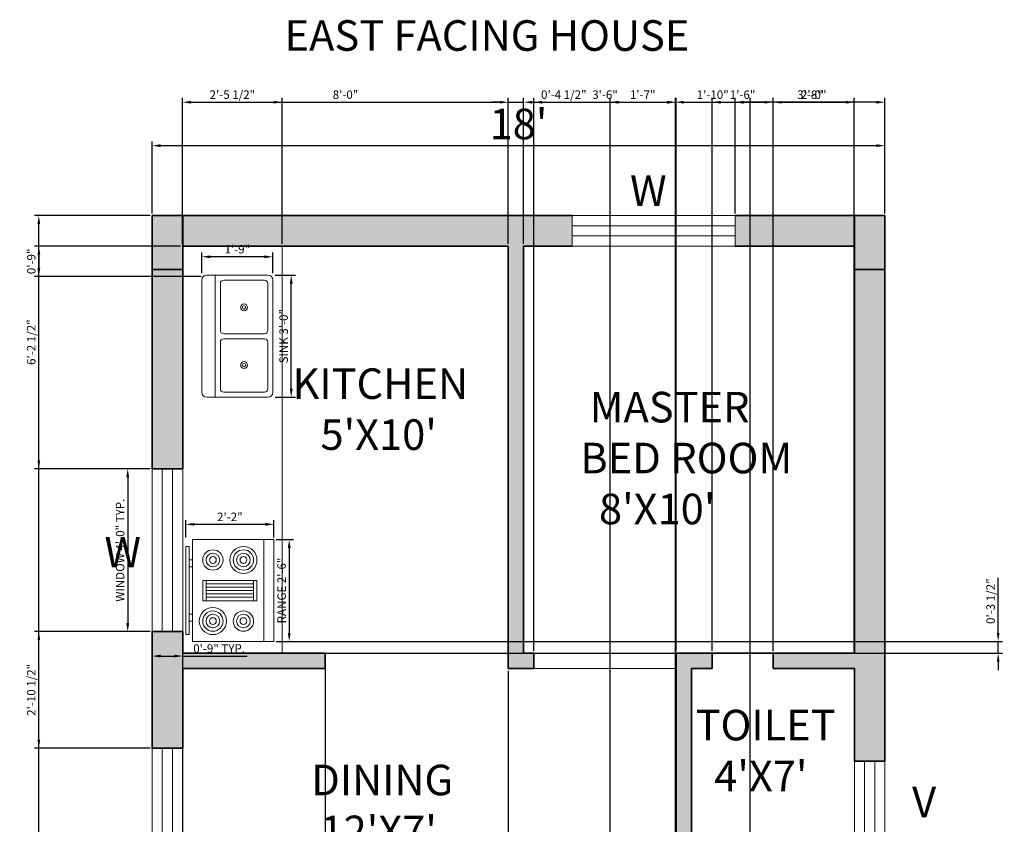
# Model space of a CAD drawing. Units: inches. Extents: x 4888 to 5178, y 5041 to 5743.
# Tile 3 of 3: x 4888 to 5178, y 5506 to 5743. Entities that reach past the tile are written whole.
import ezdxf

# ---------------------------------------------------------------- set-up
doc = ezdxf.new("R2010")
doc.units = ezdxf.units.IN
for name, color, linetype, lineweight in [('A-ANNO-DIMS', 2, 'Continuous', 18), ('A-ANNO-TEXT', 7, 'Continuous', 18), ('A-AREA-IDEN', 7, 'Continuous', 18), ('A-COLS', 7, 'Continuous', 35), ('A-DOOR', 4, 'Continuous', 18), ('A-EQPM', 9, 'Continuous', 18), ('A-FLOR-CASE', 9, 'Continuous', 18), ('A-FLOR-FIXT', 9, 'Continuous', 18), ('A-WALL', 7, 'Continuous', 35), ('A-WALL-PATT', 8, 'Continuous', 13)]:
    doc.layers.add(name, color=color, linetype=linetype, lineweight=lineweight)
doc.layers.add('A-COLS-PATT', color=18, linetype='Continuous', lineweight=13, true_color=0x000000)
doc.layers.add('A-GLAZ', color=31, linetype='Continuous', lineweight=18, true_color=0xfecc66)
doc.styles.get("Standard").update_dxf_attribs({"font": 'arial.ttf'})
doc.dimstyles.new('ISO-25', dxfattribs={"dimtxt": 2.5, "dimasz": 2.5, "dimexe": 1.25, "dimexo": 0.625, "dimtad": 1, "dimlunit": 3, "dimtxsty": 'Standard', "dimcen": 2.5, "dimadec": 0, "dimazin": 0, "dimtfac": 1, "dimtmove": 0, "dimatfit": 3, "dimfxl": 1, "dimarcsym": 0})

# ---------------------------------------------------------------- blocks, each defined once
blk = doc.blocks.new('*D1')
at = {"layer": 'A-ANNO-DIMS', "color": 0, "lineweight": -2, "transparency": 16777216}
for p, q in [((4926.84, 5685.63), (4926.84, 5706.86)), ((5142.84, 5685.63), (5142.84, 5706.86)), ((4929.34, 5705.61), (5140.34, 5705.61))]:
    blk.add_line(p, q, dxfattribs=at)
at = {"layer": 'A-ANNO-DIMS', "color": 0, "transparency": 16777216}
for points in [[(4929.34, 5706.02), (4929.34, 5705.19), (4926.84, 5705.61)], [(5140.34, 5706.02), (5140.34, 5705.19), (5142.84, 5705.61)]]:
    blk.add_solid(points, dxfattribs=at)
at = {"layer": 'Defpoints', "color": 0, "transparency": 16777216}
for p in [(5142.84, 5705.61), (4926.84, 5685.01), (5142.84, 5685.01)]:
    blk.add_point(p, dxfattribs=at)
at = {"layer": 'A-ANNO-DIMS', "color": 0, "transparency": 16777216, "insert": (5034.84, 5710.83), "char_height": 9, "attachment_point": 5}
blk.add_mtext("18'", dxfattribs=at)
blk = doc.blocks.new('Range-Oven - 30 in top')
for p, q in [((0, -3), (30, -3)), ((12, -6), (18, -6)), ((13, -20), (13, -6)), ((14, -6), (14, -20)), ((15, -20), (15, -6)), ((16, -6), (16, -20)), ((17, -20), (17, -6)), ((18, -20), (12, -20)), ((6, -24), (6, -25)), ((8, -25), (8, -24)), ((22, -25), (22, -24)), ((24, -24), (24, -25))]:
    blk.add_line(p, q)
for points in [[(0, -24), (0, 0), (30, 0), (30, -24)], [(12, -21), (12, -5), (18, -5), (18, -21)], [(2, -26), (2, -25), (28, -25), (28, -26)]]:
    blk.add_lwpolyline(points, close=True)
for centre, radius in [((6, -9), 4), ((6, -9), 3), ((6, -9), 2), ((6, -9), 1), ((24, -9), 3), ((24, -9), 2), ((24, -9), 1), ((24, -18), 4), ((6, -18), 3), ((6, -18), 2), ((6, -18), 1), ((24, -18), 3), ((24, -18), 2), ((24, -18), 1)]:
    blk.add_circle(centre, radius)
blk = doc.blocks.new('Sink-double - 36 in top')
for p, q in [((-18, -4), (18, -4)), ((-0.75, -18.5), (-0.75, -6.5)), ((0.75, -6.5), (0.75, -18.5))]:
    blk.add_line(p, q)
for points in [[(-16.5, 0), (16.5, 0)], [(-18, -19.5), (-18, -1.5)], [(18, -1.5), (18, -19.5)], [(-15.5, -5.5), (-1.75, -5.5)], [(1.75, -5.5), (15.5, -5.5)], [(-16.5, -18.5), (-16.5, -6.5)], [(16.5, -6.5), (16.5, -18.5)], [(-1.75, -19.5), (-15.5, -19.5)], [(15.5, -19.5), (1.75, -19.5)], [(16.5, -21), (-16.5, -21)]]:
    blk.add_lwpolyline(points)
for centre, radius in [((-8.5, -12.5), 1), ((8.5, -12.5), 1), ((-8.5, -12.5), 0.5), ((8.5, -12.5), 0.5)]:
    blk.add_circle(centre, radius)
for centre, radius, start, end in [((-16.5, -1.5), 1.5, 90, 180), ((16.5, -1.5), 1.5, 0, 90), ((-15.5, -6.5), 1, 90, 180), ((-1.75, -6.5), 1, 0, 90), ((1.75, -6.5), 1, 90, 180), ((15.5, -6.5), 1, 0, 90), ((-16.5, -19.5), 1.5, 180, 270), ((-15.5, -18.5), 1, 180, 270), ((-1.75, -18.5), 1, 270, 0), ((1.75, -18.5), 1, 180, 270), ((15.5, -18.5), 1, 270, 0), ((16.5, -19.5), 1.5, 270, 0)]:
    blk.add_arc(centre, radius, start, end)
blk = doc.blocks.new('WIN-48IN')
for p, q in [((0, 9), (0, 0)), ((48, 9), (0, 9)), ((48, 0), (48, 9)), ((48, 6), (0, 6)), ((48, 3), (0, 3)), ((0, 0), (48, 0))]:
    blk.add_line(p, q)
blk = doc.blocks.new('VENT-24IN')
for p, q in [((0, 24), (0, 0)), ((9, 24), (0, 24)), ((3, 0), (3, 24)), ((6, 0), (6, 24)), ((9, 0), (9, 24)), ((0, 0), (9, 0))]:
    blk.add_line(p, q)
blk = doc.blocks.new('*D7')
at = {"layer": 'A-ANNO-DIMS', "color": 0, "lineweight": -2, "transparency": 16777216}
for p, q in [((4926.22, 5610.4), (4918.39, 5610.4)), ((4919.64, 5607.9), (4919.64, 5564.9)), ((4926.22, 5562.4), (4918.39, 5562.4))]:
    blk.add_line(p, q, dxfattribs=at)
at = {"layer": 'A-ANNO-DIMS', "color": 0, "transparency": 16777216}
for points in [[(4919.23, 5607.9), (4920.06, 5607.9), (4919.64, 5610.4)], [(4919.23, 5564.9), (4920.06, 5564.9), (4919.64, 5562.4)]]:
    blk.add_solid(points, dxfattribs=at)
at = {"layer": 'Defpoints', "color": 0, "transparency": 16777216}
for p in [(4926.84, 5610.4), (4919.64, 5562.4), (4926.84, 5562.4)]:
    blk.add_point(p, dxfattribs=at)
at = {"layer": 'A-ANNO-DIMS', "color": 0, "transparency": 16777216, "insert": (4917.73, 5586.4), "char_height": 2.5, "attachment_point": 5, "rotation": 90}
blk.add_mtext('WINDOW 4\'-0" TYP.', dxfattribs=at)
blk = doc.blocks.new('*D8')
at = {"layer": 'A-ANNO-DIMS', "color": 0, "lineweight": -2, "transparency": 16777216}
for p, q in [((4926.84, 5561.78), (4926.84, 5553.95)), ((4935.84, 5561.78), (4935.84, 5553.95)), ((4929.34, 5555.2), (4933.34, 5555.2)), ((4935.84, 5555.2), (4954.83, 5555.2))]:
    blk.add_line(p, q, dxfattribs=at)
at = {"layer": 'A-ANNO-DIMS', "color": 0, "transparency": 16777216}
for points in [[(4929.34, 5555.62), (4929.34, 5554.78), (4926.84, 5555.2)], [(4933.34, 5555.62), (4933.34, 5554.78), (4935.84, 5555.2)]]:
    blk.add_solid(points, dxfattribs=at)
at = {"layer": 'Defpoints', "color": 0, "transparency": 16777216}
for p in [(4926.84, 5562.4), (4935.84, 5562.4), (4935.84, 5555.2)]:
    blk.add_point(p, dxfattribs=at)
at = {"layer": 'A-ANNO-DIMS', "color": 0, "transparency": 16777216, "insert": (4946.59, 5557.1), "char_height": 2.5, "attachment_point": 5}
blk.add_mtext('0\'-9" TYP.', dxfattribs=at)
blk = doc.blocks.new('*D13')
at = {"layer": 'A-ANNO-DIMS', "color": 0, "lineweight": -2, "transparency": 16777216}
for p, q in [((4963.38, 5589.52), (4968.5, 5589.52)), ((4967.25, 5587.02), (4967.25, 5562.02)), ((4963.38, 5559.52), (4968.5, 5559.52))]:
    blk.add_line(p, q, dxfattribs=at)
at = {"layer": 'A-ANNO-DIMS', "color": 0, "transparency": 16777216}
for points in [[(4966.83, 5587.02), (4967.67, 5587.02), (4967.25, 5589.52)], [(4966.83, 5562.02), (4967.67, 5562.02), (4967.25, 5559.52)]]:
    blk.add_solid(points, dxfattribs=at)
at = {"layer": 'Defpoints', "color": 0, "transparency": 16777216}
for p in [(4962.75, 5589.52), (4962.75, 5559.52), (4967.25, 5559.52)]:
    blk.add_point(p, dxfattribs=at)
at = {"layer": 'A-ANNO-DIMS', "color": 0, "transparency": 16777216, "insert": (4965.33, 5574.52), "char_height": 2.5, "attachment_point": 5, "rotation": 90}
blk.add_mtext('RANGE 2\'-6"', dxfattribs=at)
blk = doc.blocks.new('*D14')
at = {"layer": 'A-ANNO-DIMS', "color": 0, "lineweight": -2, "transparency": 16777216}
for p, q in [((4936.75, 5590.14), (4936.75, 5595.27)), ((4939.25, 5594.02), (4960.25, 5594.02)), ((4962.75, 5590.14), (4962.75, 5595.27))]:
    blk.add_line(p, q, dxfattribs=at)
at = {"layer": 'A-ANNO-DIMS', "color": 0, "transparency": 16777216}
for points in [[(4939.25, 5594.43), (4939.25, 5593.6), (4936.75, 5594.02)], [(4960.25, 5594.43), (4960.25, 5593.6), (4962.75, 5594.02)]]:
    blk.add_solid(points, dxfattribs=at)
at = {"layer": 'Defpoints', "color": 0, "transparency": 16777216}
for p in [(4962.75, 5594.02), (4936.75, 5589.52), (4962.75, 5589.52)]:
    blk.add_point(p, dxfattribs=at)
at = {"layer": 'A-ANNO-DIMS', "color": 0, "transparency": 16777216, "insert": (4949.75, 5595.9), "char_height": 2.5, "attachment_point": 5}
blk.add_mtext('2\'-2"', dxfattribs=at)
blk = doc.blocks.new('*D15')
at = {"layer": 'A-ANNO-DIMS', "color": 0, "lineweight": -2, "transparency": 16777216}
for p, q in [((4963.07, 5667.46), (4969.1, 5667.46)), ((4967.85, 5633.96), (4967.85, 5664.96)), ((4963.07, 5631.46), (4969.1, 5631.46))]:
    blk.add_line(p, q, dxfattribs=at)
at = {"layer": 'A-ANNO-DIMS', "color": 0, "transparency": 16777216}
for points in [[(4967.43, 5664.96), (4968.26, 5664.96), (4967.85, 5667.46)], [(4967.43, 5633.96), (4968.26, 5633.96), (4967.85, 5631.46)]]:
    blk.add_solid(points, dxfattribs=at)
at = {"layer": 'Defpoints', "color": 0, "transparency": 16777216}
for p in [(4962.45, 5667.46), (4967.85, 5667.46), (4962.45, 5631.46)]:
    blk.add_point(p, dxfattribs=at)
at = {"layer": 'A-ANNO-DIMS', "color": 0, "transparency": 16777216, "insert": (4965.93, 5649.46), "char_height": 2.5, "attachment_point": 5, "rotation": 90}
blk.add_mtext('SINK 3\'-0"', dxfattribs=at)
blk = doc.blocks.new('*D16')
at = {"layer": 'A-ANNO-DIMS', "color": 0, "lineweight": -2, "transparency": 16777216}
for p, q in [((4941.45, 5668.08), (4941.45, 5674.11)), ((4959.95, 5672.86), (4943.95, 5672.86)), ((4962.45, 5668.08), (4962.45, 5674.11))]:
    blk.add_line(p, q, dxfattribs=at)
at = {"layer": 'A-ANNO-DIMS', "color": 0, "transparency": 16777216}
for points in [[(4943.95, 5673.27), (4943.95, 5672.44), (4941.45, 5672.86)], [(4959.95, 5673.27), (4959.95, 5672.44), (4962.45, 5672.86)]]:
    blk.add_solid(points, dxfattribs=at)
at = {"layer": 'Defpoints', "color": 0, "transparency": 16777216}
for p in [(4941.45, 5672.86), (4941.45, 5667.46), (4962.45, 5667.46)]:
    blk.add_point(p, dxfattribs=at)
at = {"layer": 'A-ANNO-DIMS', "color": 0, "transparency": 16777216, "insert": (4951.95, 5674.76), "char_height": 2.5, "attachment_point": 5}
blk.add_mtext('1\'-9"', dxfattribs=at)
blk = doc.blocks.new('*D17')
at = {"layer": 'A-ANNO-DIMS', "color": 0, "lineweight": -2, "transparency": 16777216}
for p, q in [((4926.22, 5685.01), (4892.19, 5685.01)), ((4893.44, 5078.51), (4893.44, 5682.51)), ((4926.22, 5076.01), (4892.19, 5076.01))]:
    blk.add_line(p, q, dxfattribs=at)
at = {"layer": 'A-ANNO-DIMS', "color": 0, "transparency": 16777216}
for points in [[(4893.03, 5682.51), (4893.86, 5682.51), (4893.44, 5685.01)], [(4893.03, 5078.51), (4893.86, 5078.51), (4893.44, 5076.01)]]:
    blk.add_solid(points, dxfattribs=at)
at = {"layer": 'Defpoints', "color": 0, "transparency": 16777216}
for p in [(4893.44, 5685.01), (4926.84, 5685.01), (4926.84, 5076.01)]:
    blk.add_point(p, dxfattribs=at)
at = {"layer": 'A-ANNO-DIMS', "color": 0, "transparency": 16777216, "insert": (4891.54, 5380.51), "char_height": 2.5, "attachment_point": 5, "rotation": 90}
blk.add_mtext('50\'-9"', dxfattribs=at)
blk = doc.blocks.new('*D18')
at = {"layer": 'A-ANNO-DIMS', "color": 0, "lineweight": -2, "transparency": 16777216}
for p, q in [((5098.68, 5685.63), (5098.68, 5719.66)), ((5140.34, 5718.41), (5101.18, 5718.41)), ((5142.84, 5685.63), (5142.84, 5719.66))]:
    blk.add_line(p, q, dxfattribs=at)
at = {"layer": 'A-ANNO-DIMS', "color": 0, "transparency": 16777216}
for points in [[(5101.18, 5718.82), (5101.18, 5717.99), (5098.68, 5718.41)], [(5140.34, 5718.82), (5140.34, 5717.99), (5142.84, 5718.41)]]:
    blk.add_solid(points, dxfattribs=at)
at = {"layer": 'Defpoints', "color": 0, "transparency": 16777216}
for p in [(5098.68, 5718.41), (5098.68, 5685.01), (5142.84, 5685.01)]:
    blk.add_point(p, dxfattribs=at)
at = {"layer": 'A-ANNO-DIMS', "color": 0, "transparency": 16777216, "insert": (5120.76, 5720.31), "char_height": 2.5, "attachment_point": 5}
blk.add_mtext('3\'-8"', dxfattribs=at)
blk = doc.blocks.new('*D19')
at = {"layer": 'A-ANNO-DIMS', "color": 0, "lineweight": -2, "transparency": 16777216}
for p, q in [((4926.22, 5685.01), (4892.19, 5685.01)), ((4893.44, 5612.9), (4893.44, 5682.51)), ((4926.22, 5610.4), (4892.19, 5610.4))]:
    blk.add_line(p, q, dxfattribs=at)
at = {"layer": 'A-ANNO-DIMS', "color": 0, "transparency": 16777216}
for points in [[(4893.03, 5682.51), (4893.86, 5682.51), (4893.44, 5685.01)], [(4893.03, 5612.9), (4893.86, 5612.9), (4893.44, 5610.4)]]:
    blk.add_solid(points, dxfattribs=at)
at = {"layer": 'Defpoints', "color": 0, "transparency": 16777216}
for p in [(4893.44, 5685.01), (4926.84, 5685.01), (4926.84, 5610.4)]:
    blk.add_point(p, dxfattribs=at)
at = {"layer": 'A-ANNO-DIMS', "color": 0, "transparency": 16777216, "insert": (4891.53, 5647.7), "char_height": 2.5, "attachment_point": 5, "rotation": 90}
blk.add_mtext('6\'-2 1/2"', dxfattribs=at)
blk = doc.blocks.new('*D20')
at = {"layer": 'A-ANNO-DIMS', "color": 0, "lineweight": -2, "transparency": 16777216}
for p, q in [((4926.22, 5562.4), (4892.19, 5562.4)), ((4893.44, 5530.6), (4893.44, 5559.9)), ((4926.22, 5528.1), (4892.19, 5528.1))]:
    blk.add_line(p, q, dxfattribs=at)
at = {"layer": 'A-ANNO-DIMS', "color": 0, "transparency": 16777216}
for points in [[(4893.03, 5559.9), (4893.86, 5559.9), (4893.44, 5562.4)], [(4893.03, 5530.6), (4893.86, 5530.6), (4893.44, 5528.1)]]:
    blk.add_solid(points, dxfattribs=at)
at = {"layer": 'Defpoints', "color": 0, "transparency": 16777216}
for p in [(4893.44, 5562.4), (4926.84, 5562.4), (4926.84, 5528.1)]:
    blk.add_point(p, dxfattribs=at)
at = {"layer": 'A-ANNO-DIMS', "color": 0, "transparency": 16777216, "insert": (4891.53, 5545.25), "char_height": 2.5, "attachment_point": 5, "rotation": 90}
blk.add_mtext('2\'-10 1/2"', dxfattribs=at)
blk = doc.blocks.new('*D32')
at = {"layer": 'A-ANNO-DIMS', "color": 0, "lineweight": -2, "transparency": 16777216}
for p, q in [((4977.89, 5550.88), (4977.89, 5041.36)), ((5031.84, 5550.88), (5031.84, 5041.36)), ((4980.39, 5042.61), (5029.34, 5042.61))]:
    blk.add_line(p, q, dxfattribs=at)
at = {"layer": 'A-ANNO-DIMS', "color": 0, "transparency": 16777216}
for points in [[(4980.39, 5043.02), (4980.39, 5042.19), (4977.89, 5042.61)], [(5029.34, 5043.02), (5029.34, 5042.19), (5031.84, 5042.61)]]:
    blk.add_solid(points, dxfattribs=at)
at = {"layer": 'Defpoints', "color": 0, "transparency": 16777216}
for p in [(4977.89, 5551.51), (5031.84, 5551.51), (5031.84, 5042.61)]:
    blk.add_point(p, dxfattribs=at)
at = {"layer": 'A-ANNO-DIMS', "color": 0, "transparency": 16777216, "insert": (5004.87, 5044.51), "char_height": 2.5, "attachment_point": 5}
blk.add_mtext('4\'-6"', dxfattribs=at)
blk = doc.blocks.new('*D33')
at = {"layer": 'A-ANNO-DIMS', "color": 0, "lineweight": -2, "transparency": 16777216}
for p, q in [((5039.34, 5556.63), (5039.34, 5719.66)), ((5041.84, 5718.41), (5078.84, 5718.41)), ((5081.34, 5556.63), (5081.34, 5719.66))]:
    blk.add_line(p, q, dxfattribs=at)
at = {"layer": 'A-ANNO-DIMS', "color": 0, "transparency": 16777216}
for points in [[(5041.84, 5718.82), (5041.84, 5717.99), (5039.34, 5718.41)], [(5078.84, 5718.82), (5078.84, 5717.99), (5081.34, 5718.41)]]:
    blk.add_solid(points, dxfattribs=at)
at = {"layer": 'Defpoints', "color": 0, "transparency": 16777216}
for p in [(5081.34, 5718.41), (5039.34, 5556.01), (5081.34, 5556.01)]:
    blk.add_point(p, dxfattribs=at)
at = {"layer": 'A-ANNO-DIMS', "color": 0, "transparency": 16777216, "insert": (5060.34, 5720.31), "char_height": 2.5, "attachment_point": 5}
blk.add_mtext('3\'-6"', dxfattribs=at)
blk = doc.blocks.new('*D34')
at = {"layer": 'A-ANNO-DIMS', "color": 0, "lineweight": -2, "transparency": 16777216}
for p, q in [((5091.9, 5556.63), (5091.9, 5719.66)), ((5094.4, 5718.41), (5107.4, 5718.41)), ((5109.9, 5556.63), (5109.9, 5719.66))]:
    blk.add_line(p, q, dxfattribs=at)
at = {"layer": 'A-ANNO-DIMS', "color": 0, "transparency": 16777216}
for points in [[(5094.4, 5718.82), (5094.4, 5717.99), (5091.9, 5718.41)], [(5107.4, 5718.82), (5107.4, 5717.99), (5109.9, 5718.41)]]:
    blk.add_solid(points, dxfattribs=at)
at = {"layer": 'Defpoints', "color": 0, "transparency": 16777216}
for p in [(5109.9, 5718.41), (5091.9, 5556.01), (5109.9, 5556.01)]:
    blk.add_point(p, dxfattribs=at)
at = {"layer": 'A-ANNO-DIMS', "color": 0, "transparency": 16777216, "insert": (5100.9, 5720.31), "char_height": 2.5, "attachment_point": 5}
blk.add_mtext('1\'-6"', dxfattribs=at)
blk = doc.blocks.new('*D35')
at = {"layer": 'A-ANNO-DIMS', "color": 0, "lineweight": -2, "transparency": 16777216}
for p, q in [((5109.9, 5556.63), (5109.9, 5719.66)), ((5112.4, 5718.41), (5131.34, 5718.41)), ((5133.84, 5556.63), (5133.84, 5719.66))]:
    blk.add_line(p, q, dxfattribs=at)
at = {"layer": 'A-ANNO-DIMS', "color": 0, "transparency": 16777216}
for points in [[(5112.4, 5718.82), (5112.4, 5717.99), (5109.9, 5718.41)], [(5131.34, 5718.82), (5131.34, 5717.99), (5133.84, 5718.41)]]:
    blk.add_solid(points, dxfattribs=at)
at = {"layer": 'Defpoints', "color": 0, "transparency": 16777216}
for p in [(5133.84, 5718.41), (5109.9, 5556.01), (5133.84, 5556.01)]:
    blk.add_point(p, dxfattribs=at)
at = {"layer": 'A-ANNO-DIMS', "color": 0, "transparency": 16777216, "insert": (5121.87, 5720.31), "char_height": 2.5, "attachment_point": 5}
blk.add_mtext('2\'-0"', dxfattribs=at)
blk = doc.blocks.new('*D36')
at = {"layer": 'A-ANNO-DIMS', "color": 0, "lineweight": -2, "transparency": 16777216}
for p, q in [((5081.08, 5204.13), (5081.08, 5719.66)), ((5083.58, 5718.41), (5100.61, 5718.41)), ((5103.11, 5204.13), (5103.11, 5719.66))]:
    blk.add_line(p, q, dxfattribs=at)
at = {"layer": 'A-ANNO-DIMS', "color": 0, "transparency": 16777216}
for points in [[(5083.58, 5718.82), (5083.58, 5717.99), (5081.08, 5718.41)], [(5100.61, 5718.82), (5100.61, 5717.99), (5103.11, 5718.41)]]:
    blk.add_solid(points, dxfattribs=at)
at = {"layer": 'Defpoints', "color": 0, "transparency": 16777216}
for p in [(5103.11, 5718.41), (5081.08, 5203.51), (5103.11, 5203.51)]:
    blk.add_point(p, dxfattribs=at)
at = {"layer": 'A-ANNO-DIMS', "color": 0, "transparency": 16777216, "insert": (5092.09, 5720.31), "char_height": 2.5, "attachment_point": 5}
blk.add_mtext('1\'-10"', dxfattribs=at)
blk = doc.blocks.new('*D38')
at = {"layer": 'A-ANNO-DIMS', "color": 0, "lineweight": -2, "transparency": 16777216}
for p, q in [((4935.84, 5676.63), (4935.84, 5719.66)), ((4938.34, 5718.41), (4962.66, 5718.41)), ((4965.16, 5676.63), (4965.16, 5719.66))]:
    blk.add_line(p, q, dxfattribs=at)
at = {"layer": 'A-ANNO-DIMS', "color": 0, "transparency": 16777216}
for points in [[(4938.34, 5718.82), (4938.34, 5717.99), (4935.84, 5718.41)], [(4962.66, 5718.82), (4962.66, 5717.99), (4965.16, 5718.41)]]:
    blk.add_solid(points, dxfattribs=at)
at = {"layer": 'Defpoints', "color": 0, "transparency": 16777216}
for p in [(4965.16, 5718.41), (4935.84, 5676.01), (4965.16, 5676.01)]:
    blk.add_point(p, dxfattribs=at)
at = {"layer": 'A-ANNO-DIMS', "color": 0, "transparency": 16777216, "insert": (4950.5, 5720.32), "char_height": 2.5, "attachment_point": 5}
blk.add_mtext('2\'-5 1/2"', dxfattribs=at)
blk = doc.blocks.new('*D39')
at = {"layer": 'A-ANNO-DIMS', "color": 0, "lineweight": -2, "transparency": 16777216}
for p, q in [((4935.84, 5555.38), (4935.84, 5041.36)), ((4977.89, 5555.38), (4977.89, 5041.36)), ((4938.34, 5042.61), (4975.39, 5042.61))]:
    blk.add_line(p, q, dxfattribs=at)
at = {"layer": 'A-ANNO-DIMS', "color": 0, "transparency": 16777216}
for points in [[(4938.34, 5043.02), (4938.34, 5042.19), (4935.84, 5042.61)], [(4975.39, 5043.02), (4975.39, 5042.19), (4977.89, 5042.61)]]:
    blk.add_solid(points, dxfattribs=at)
at = {"layer": 'Defpoints', "color": 0, "transparency": 16777216}
for p in [(4935.84, 5556.01), (4977.89, 5556.01), (4977.89, 5042.61)]:
    blk.add_point(p, dxfattribs=at)
at = {"layer": 'A-ANNO-DIMS', "color": 0, "transparency": 16777216, "insert": (4956.87, 5044.51), "char_height": 2.5, "attachment_point": 5}
blk.add_mtext('3\'-6"', dxfattribs=at)
blk = doc.blocks.new('*D40')
at = {"layer": 'A-ANNO-DIMS', "color": 0, "lineweight": -2, "transparency": 16777216}
for p, q in [((5061.84, 5204.13), (5061.84, 5719.66)), ((5064.34, 5718.41), (5078.58, 5718.41)), ((5081.08, 5204.13), (5081.08, 5719.66))]:
    blk.add_line(p, q, dxfattribs=at)
at = {"layer": 'A-ANNO-DIMS', "color": 0, "transparency": 16777216}
for points in [[(5064.34, 5718.82), (5064.34, 5717.99), (5061.84, 5718.41)], [(5078.58, 5718.82), (5078.58, 5717.99), (5081.08, 5718.41)]]:
    blk.add_solid(points, dxfattribs=at)
at = {"layer": 'Defpoints', "color": 0, "transparency": 16777216}
for p in [(5081.08, 5718.41), (5061.84, 5203.51), (5081.08, 5203.51)]:
    blk.add_point(p, dxfattribs=at)
at = {"layer": 'A-ANNO-DIMS', "color": 0, "transparency": 16777216, "insert": (5071.46, 5720.29), "char_height": 2.5, "attachment_point": 5}
blk.add_mtext('1\'-7"', dxfattribs=at)
blk = doc.blocks.new('*D42')
at = {"layer": 'A-ANNO-DIMS', "color": 0, "lineweight": -2, "transparency": 16777216}
for p, q in [((4935.22, 5676.01), (4892.19, 5676.01)), ((4893.44, 5673.51), (4893.44, 5669.52)), ((4941.26, 5667.02), (4892.19, 5667.02))]:
    blk.add_line(p, q, dxfattribs=at)
at = {"layer": 'A-ANNO-DIMS', "color": 0, "transparency": 16777216}
for points in [[(4893.03, 5673.51), (4893.86, 5673.51), (4893.44, 5676.01)], [(4893.03, 5669.52), (4893.86, 5669.52), (4893.44, 5667.02)]]:
    blk.add_solid(points, dxfattribs=at)
at = {"layer": 'Defpoints', "color": 0, "transparency": 16777216}
for p in [(4935.84, 5676.01), (4893.44, 5667.02), (4941.88, 5667.02)]:
    blk.add_point(p, dxfattribs=at)
at = {"layer": 'A-ANNO-DIMS', "color": 0, "transparency": 16777216, "insert": (4891.54, 5671.51), "char_height": 2.5, "attachment_point": 5, "rotation": 90}
blk.add_mtext('0\'-9"', dxfattribs=at)
blk = doc.blocks.new('*D43')
at = {"layer": 'A-ANNO-DIMS', "color": 0, "lineweight": -2, "transparency": 16777216}
for p, q in [((5176.24, 5562.02), (5176.24, 5578.24)), ((4963.38, 5559.52), (5177.49, 5559.52)), ((5176.24, 5556.01), (5176.24, 5559.52)), ((4965.79, 5556.01), (5177.49, 5556.01)), ((5176.24, 5553.51), (5176.24, 5551.01))]:
    blk.add_line(p, q, dxfattribs=at)
at = {"layer": 'A-ANNO-DIMS', "color": 0, "transparency": 16777216}
for points in [[(5175.83, 5562.02), (5176.66, 5562.02), (5176.24, 5559.52)], [(5175.83, 5553.51), (5176.66, 5553.51), (5176.24, 5556.01)]]:
    blk.add_solid(points, dxfattribs=at)
at = {"layer": 'Defpoints', "color": 0, "transparency": 16777216}
for p in [(4962.75, 5559.52), (5176.24, 5559.52), (4965.16, 5556.01)]:
    blk.add_point(p, dxfattribs=at)
at = {"layer": 'A-ANNO-DIMS', "color": 0, "transparency": 16777216, "insert": (5174.33, 5571.38), "char_height": 2.5, "attachment_point": 5, "rotation": 90}
blk.add_mtext('0\'-3 1/2"', dxfattribs=at)
blk = doc.blocks.new('*D44')
at = {"layer": 'A-ANNO-DIMS', "color": 0, "lineweight": -2, "transparency": 16777216}
for p, q in [((5029.34, 5718.41), (5026.84, 5718.41)), ((5031.84, 5676.63), (5031.84, 5719.66)), ((5031.84, 5718.41), (5036.34, 5718.41)), ((5036.34, 5676.63), (5036.34, 5719.66)), ((5038.84, 5718.41), (5055.06, 5718.41))]:
    blk.add_line(p, q, dxfattribs=at)
at = {"layer": 'A-ANNO-DIMS', "color": 0, "transparency": 16777216}
for points in [[(5029.34, 5718.82), (5029.34, 5717.99), (5031.84, 5718.41)], [(5038.84, 5718.82), (5038.84, 5717.99), (5036.34, 5718.41)]]:
    blk.add_solid(points, dxfattribs=at)
at = {"layer": 'Defpoints', "color": 0, "transparency": 16777216}
for p in [(5036.34, 5718.41), (5031.84, 5676.01), (5036.34, 5676.01)]:
    blk.add_point(p, dxfattribs=at)
at = {"layer": 'A-ANNO-DIMS', "color": 0, "transparency": 16777216, "insert": (5048.2, 5720.32), "char_height": 2.5, "attachment_point": 5}
blk.add_mtext('0\'-4 1/2"', dxfattribs=at)
blk = doc.blocks.new('*D49')
at = {"layer": 'A-ANNO-DIMS', "color": 0, "lineweight": -2, "transparency": 16777216}
for p, q in [((4935.84, 5676.63), (4935.84, 5719.66)), ((4938.34, 5718.41), (5029.34, 5718.41)), ((5031.84, 5676.63), (5031.84, 5719.66))]:
    blk.add_line(p, q, dxfattribs=at)
at = {"layer": 'A-ANNO-DIMS', "color": 0, "transparency": 16777216}
for points in [[(4938.34, 5718.82), (4938.34, 5717.99), (4935.84, 5718.41)], [(5029.34, 5718.82), (5029.34, 5717.99), (5031.84, 5718.41)]]:
    blk.add_solid(points, dxfattribs=at)
at = {"layer": 'Defpoints', "color": 0, "transparency": 16777216}
for p in [(5031.84, 5718.41), (4935.84, 5676.01), (5031.84, 5676.01)]:
    blk.add_point(p, dxfattribs=at)
at = {"layer": 'A-ANNO-DIMS', "color": 0, "transparency": 16777216, "insert": (4983.84, 5720.31), "char_height": 2.5, "attachment_point": 5}
blk.add_mtext('8\'-0"', dxfattribs=at)

msp = doc.modelspace()

# ---------------------------------------------------------------- hatches: boundary and pattern name
at = {"layer": 'A-COLS-PATT'}
h = msp.add_hatch(color=256, dxfattribs=at)
h.dxf.hatch_style = 1
h.paths.add_polyline_path([(4935.844, 5685.006), (4926.844, 5685.006), (4926.844, 5669.086), (4935.844, 5669.086)])
h.paths.add_polyline_path([(5142.844, 5685.006), (5133.844, 5685.006), (5133.844, 5669.086), (5142.844, 5669.086)])
h.paths.add_polyline_path([(4935.844, 5467.506), (4926.844, 5467.506), (4926.844, 5455.506), (4926.844, 5446.68), (4935.844, 5446.68)])
h.paths.add_polyline_path([(5142.844, 5467.506), (5133.844, 5467.506), (5133.844, 5446.68), (5142.844, 5446.68)])
h.paths.add_polyline_path([(4935.844, 5340.228), (4926.844, 5340.228), (4926.844, 5313.351), (4935.844, 5313.351)])
h.paths.add_polyline_path([(4935.844, 5095.626), (4926.844, 5095.626), (4926.844, 5076.006), (4935.844, 5076.006)])
h.paths.add_polyline_path([(5142.844, 5095.626), (5133.844, 5095.626), (5133.844, 5076.006), (5142.844, 5076.006)])
at = {"layer": 'A-WALL-PATT'}
h = msp.add_hatch(color=256, dxfattribs=at)
h.dxf.hatch_style = 1
h.paths.add_polyline_path([(5050.684, 5685.006), (4935.844, 5685.006), (4935.844, 5676.006), (5031.844, 5676.006), (5031.844, 5551.506), (5039.344, 5551.506), (5039.344, 5556.006), (5036.344, 5556.006), (5036.344, 5676.006), (5050.684, 5676.006)])
h.paths.add_polyline_path([(4935.844, 5669.086), (4926.844, 5669.086), (4926.844, 5610.401), (4935.844, 5610.401)])
h.paths.add_polyline_path([(5133.844, 5685.006), (5098.684, 5685.006), (5098.684, 5676.006), (5133.844, 5676.006)])
h.paths.add_polyline_path([(5142.844, 5669.086), (5133.844, 5669.086), (5133.844, 5556.006), (5109.899, 5556.006), (5109.899, 5551.506), (5133.844, 5551.506), (5133.844, 5524.266), (5142.844, 5524.266)])
h.paths.add_polyline_path([(4977.891, 5556.006), (4935.844, 5556.006), (4935.844, 5562.401), (4926.844, 5562.401), (4926.844, 5528.1), (4935.844, 5528.1), (4935.844, 5551.506), (4977.891, 5551.506)])
h.paths.add_polyline_path([(4935.844, 5480.1), (4926.844, 5480.1), (4926.844, 5467.506), (4935.844, 5467.506)])
h.paths.add_polyline_path([(5022.844, 5467.506), (4935.844, 5467.506), (4935.844, 5463.006), (5013.844, 5463.006), (5013.844, 5388.655), (5022.844, 5388.655)])
h.paths.add_polyline_path([(5133.844, 5467.506), (5085.844, 5467.506), (5085.844, 5551.506), (5091.899, 5551.506), (5091.899, 5556.006), (5081.344, 5556.006), (5081.344, 5463.006), (5133.844, 5463.006)])
h.paths.add_polyline_path([(5142.844, 5500.266), (5133.844, 5500.266), (5133.844, 5467.506), (5142.844, 5467.506)])
h.paths.add_polyline_path([(5142.844, 5446.68), (5133.844, 5446.68), (5133.844, 5420.006), (5142.844, 5420.006)])
h.paths.add_polyline_path([(5022.844, 5323.506), (5067.366, 5323.506), (5067.366, 5328.006), (5022.844, 5328.006), (5022.844, 5340.655), (5013.844, 5340.655), (5013.844, 5137.506), (5061.844, 5137.506), (5061.844, 5122.915), (5070.844, 5122.915), (5070.844, 5137.506), (5133.844, 5137.506), (5133.844, 5119.626), (5142.844, 5119.626), (5142.844, 5158.641), (5133.844, 5158.641), (5133.844, 5146.506), (5070.844, 5146.506), (5070.844, 5194.506), (5081.079, 5194.506), (5081.079, 5203.506), (5061.844, 5203.506), (5061.844, 5146.506), (5022.844, 5146.506)])
h.paths.add_polyline_path([(4935.844, 5313.351), (4926.844, 5313.351), (4926.844, 5095.626), (4935.844, 5095.626)])
h.paths.add_polyline_path([(4935.844, 5446.68), (4926.844, 5446.68), (4926.844, 5340.228), (4935.844, 5340.228)])
h.paths.add_polyline_path([(5142.844, 5372.006), (5133.844, 5372.006), (5133.844, 5340.228), (5142.844, 5340.228)])
h.paths.add_polyline_path([(5133.844, 5328.006), (5109.366, 5328.006), (5109.366, 5323.506), (5133.844, 5323.506)], flags=17)
h.paths.add_polyline_path([(5142.844, 5313.351), (5133.844, 5313.351), (5133.844, 5282.61), (5142.844, 5282.61)], flags=17)
h.paths.add_polyline_path([(5142.844, 5234.61), (5133.844, 5234.61), (5133.844, 5203.506), (5103.109, 5203.506), (5103.109, 5194.506), (5133.844, 5194.506), (5133.844, 5182.641), (5142.844, 5182.641)], flags=17)
h.paths.add_polyline_path([(5133.844, 5085.006), (4935.844, 5085.006), (4935.844, 5076.006), (5133.844, 5076.006)])
h.paths.add_polyline_path([(5070.844, 5094.96), (5061.844, 5094.96), (5061.844, 5085.006), (5070.844, 5085.006)])

# ---------------------------------------------------------------- linework, layer by layer
at = {"layer": 'A-COLS'}
for p, q in [((4926.844, 5685.006), (4926.844, 5685.006)), ((4926.844, 5685.006), (4926.844, 5685.006)), ((4935.844, 5669.086), (4926.844, 5669.086)), ((5133.844, 5669.086), (5142.844, 5669.086))]:
    msp.add_line(p, q, dxfattribs=at)
at = {"layer": 'A-DOOR'}
msp.add_line((5081.344, 5551.506), (5039.344, 5551.506), dxfattribs=at)
at = {"layer": 'A-FLOR-CASE'}
msp.add_line((4965.164, 5556.006), (4965.164, 5676.006), dxfattribs=at)
at = {"layer": 'A-WALL'}
for p, q in [((4926.844, 5685.006), (5050.684, 5685.006)), ((4926.844, 5610.401), (4926.844, 5685.006)), ((4935.844, 5610.401), (4935.844, 5685.006)), ((5098.684, 5685.006), (5142.844, 5685.006)), ((5133.844, 5685.006), (5133.844, 5556.006)), ((5142.844, 5685.006), (5142.844, 5524.266)), ((4935.844, 5676.006), (5031.844, 5676.006)), ((5031.844, 5551.506), (5031.844, 5676.006)), ((5036.344, 5556.006), (5036.344, 5676.006)), ((5036.344, 5676.006), (5050.684, 5676.006)), ((5098.684, 5676.006), (5133.844, 5676.006)), ((4926.844, 5610.401), (4935.844, 5610.401)), ((4926.844, 5562.401), (4935.844, 5562.401)), ((4926.844, 5528.1), (4926.844, 5562.401)), ((4935.844, 5556.006), (4935.844, 5562.401)), ((4935.844, 5556.006), (4977.891, 5556.006)), ((4977.891, 5556.006), (4977.891, 5551.506)), ((5036.344, 5556.006), (5039.344, 5556.006)), ((5039.344, 5556.006), (5039.344, 5551.506)), ((5081.344, 5556.006), (5081.344, 5463.006)), ((5081.344, 5556.006), (5133.844, 5556.006)), ((5091.899, 5556.006), (5091.899, 5551.506)), ((5109.899, 5556.006), (5109.899, 5551.506)), ((4935.844, 5551.506), (4977.891, 5551.506)), ((4935.844, 5528.1), (4935.844, 5551.506)), ((5031.844, 5551.506), (5039.344, 5551.506)), ((5085.844, 5551.506), (5085.844, 5467.506)), ((5085.844, 5551.506), (5091.899, 5551.506)), ((5109.899, 5551.506), (5133.844, 5551.506)), ((5133.844, 5551.506), (5133.844, 5524.266)), ((4926.844, 5528.1), (4935.844, 5528.1)), ((5133.844, 5524.266), (5142.844, 5524.266))]:
    msp.add_line(p, q, dxfattribs=at)

# ---------------------------------------------------------------- block references
at = {"layer": 'A-EQPM', "rotation": 270}
msp.add_blockref('Range-Oven - 30 in top', (4962.751, 5589.515), dxfattribs=at)
at = {"layer": 'A-FLOR-FIXT', "rotation": 90}
msp.add_blockref('Sink-double - 36 in top', (4941.446, 5649.455), dxfattribs=at)
at = {"layer": 'A-GLAZ'}
for name, p in [('WIN-48IN', (5050.684, 5676.006)), ('VENT-24IN', (5133.844, 5500.266))]:
    msp.add_blockref(name, p, dxfattribs=at)
for p, rotation in [((4926.844, 5610.402), 270.0000000000021), ((4935.844, 5480.1), 89.9999999999992)]:
    msp.add_blockref('WIN-48IN', p, dxfattribs=dict(at, rotation=rotation))

# ---------------------------------------------------------------- texts
at = {"layer": 'A-ANNO-TEXT', "char_height": 9, "attachment_point": 1}
for s, width, heights, insert in [(' EAST FACING HOUSE', 184.74973, [72.426], (4963.134, 5742.566)), ('W', 76.41803, [0], (5067.724, 5696.822)), ('W', 76.41803, [0], (4912.776, 5590.325)), ('V', 76.41803, [0], (5150.879, 5516.666))]:
    msp.add_mtext_dynamic_manual_height_columns(s, width=width, gutter_width=12.5, heights=heights, dxfattribs=dict(at, insert=insert))
at = {"layer": 'A-AREA-IDEN', "char_height": 9, "attachment_point": 1}
for s, width, heights, insert in [(" KITCHEN\\P   5'X10'", 46.89694, [0], (4968.219, 5639.968)), (" MASTER \\PBED ROOM\\P  8'X10'", 291.65424, [93.722], (5053.07, 5633.058)), (" TOILET\\P   4'X7'", 86.29199, [67.013], (5084.293, 5539.359)), (" DINING \\P  12'X7'", 113.95373, [67.058], (4970.97, 5523.183))]:
    msp.add_mtext_dynamic_manual_height_columns(s, width=width, gutter_width=12.5, heights=heights, dxfattribs=dict(at, insert=insert))

# ---------------------------------------------------------------- dimensions: what is measured, and where the dimension line sits
at = {"layer": 'A-ANNO-DIMS'}
for base, p1, p2, override, picture, middle in [((4965.164, 5718.406), (4935.844, 5676.006), (4965.164, 5676.006), {"dimdec": 1, "dimlfac": 1, "dimrnd": 0, "dimzin": 1, "dimdsep": 46, "dimlunit": 4, "dimfrac": 2}, '*D38', (4950.504, 5720.324)), ((5036.344, 5718.406), (5031.844, 5676.006), (5036.344, 5676.006), {"dimdec": 1, "dimlfac": 1, "dimrnd": 0, "dimzin": 1, "dimdsep": 46, "dimlunit": 4, "dimfrac": 2}, '*D44', (5048.204, 5720.324)), ((5031.844, 5718.406), (4935.844, 5676.006), (5031.844, 5676.006), {"dimdec": 1, "dimlfac": 1, "dimrnd": 0, "dimzin": 1, "dimdsep": 46, "dimlunit": 4, "dimfrac": 2}, '*D49', (4983.844, 5720.307)), ((5081.344, 5718.406), (5039.344, 5556.006), (5081.344, 5556.006), {"dimdec": 1, "dimlfac": 1, "dimrnd": 0, "dimzin": 1, "dimdsep": 46, "dimlunit": 4, "dimfrac": 2}, '*D33', (5060.344, 5720.308)), ((5081.079, 5718.406), (5061.844, 5203.506), (5081.079, 5203.506), {"dimdec": 1, "dimlfac": 1, "dimrnd": 0, "dimzin": 1, "dimdsep": 46, "dimlunit": 4, "dimfrac": 2}, '*D40', (5071.462, 5720.286)), ((5103.109, 5718.406), (5081.079, 5203.506), (5103.109, 5203.506), {"dimdec": 1, "dimlfac": 1, "dimrnd": 0, "dimzin": 1, "dimdsep": 46, "dimlunit": 4, "dimfrac": 2}, '*D36', (5092.094, 5720.307)), ((5109.899, 5718.406), (5091.899, 5556.006), (5109.899, 5556.006), {"dimdec": 1, "dimlfac": 1, "dimrnd": 0, "dimzin": 1, "dimdsep": 46, "dimlunit": 4, "dimfrac": 2}, '*D34', (5100.899, 5720.307)), ((5098.684, 5718.406), (5142.844, 5685.006), (5098.684, 5685.006), {"dimdec": 1, "dimlfac": 1, "dimrnd": 0, "dimzin": 1, "dimdsep": 46, "dimlunit": 4, "dimfrac": 2}, '*D18', (5120.764, 5720.308)), ((5133.844, 5718.406), (5109.899, 5556.006), (5133.844, 5556.006), {"dimdec": 1, "dimlfac": 1, "dimrnd": 0, "dimzin": 1, "dimdsep": 46, "dimlunit": 4, "dimfrac": 2}, '*D35', (5121.871, 5720.307)), ((5142.844, 5705.606), (4926.844, 5685.006), (5142.844, 5685.006), {"dimtxt": 9, "dimclrd": 0, "dimclre": 0, "dimclrt": 0}, '*D1', (5034.844, 5710.826)), ((4962.751, 5594.015), (4936.751, 5589.515), (4962.751, 5589.515), {"dimdec": 1, "dimlfac": 1, "dimrnd": 0, "dimzin": 1, "dimdsep": 46, "dimlunit": 4, "dimfrac": 2}, '*D14', (4949.751, 5595.896)), ((4977.891, 5042.606), (4935.844, 5556.006), (4977.891, 5556.006), {"dimdec": 1, "dimlfac": 1, "dimrnd": 0, "dimzin": 1, "dimdsep": 46, "dimlunit": 4, "dimfrac": 2}, '*D39', (4956.867, 5044.508)), ((5031.844, 5042.606), (4977.891, 5551.506), (5031.844, 5551.506), {"dimdec": 1, "dimlfac": 1, "dimrnd": 0, "dimzin": 1, "dimdsep": 46, "dimlunit": 4, "dimfrac": 2}, '*D32', (5004.867, 5044.507))]:
    dim = msp.add_linear_dim(base=base, p1=p1, p2=p2, dimstyle='ISO-25', override=override, dxfattribs=at)
    dim.commit()
    dim.dimension.update_dxf_attribs({"geometry": picture, "text_midpoint": middle})
for base, p1, p2, angle, picture, middle in [((4893.444, 5685.006), (4926.844, 5610.401), (4926.844, 5685.006), 90, '*D19', (4891.526, 5647.704)), ((4893.444, 5685.006), (4926.844, 5076.006), (4926.844, 5685.006), 90, '*D17', (4891.542, 5380.506)), ((4893.444, 5667.016), (4935.844, 5676.006), (4941.885, 5667.016), 90, '*D42', (4891.542, 5671.511)), ((4941.446, 5672.855), (4962.446, 5667.455), (4941.446, 5667.455), 180, '*D16', (4951.946, 5674.757)), ((5176.244, 5559.515), (4965.164, 5556.006), (4962.751, 5559.515), 90, '*D43', (5174.325, 5571.376)), ((4893.444, 5562.401), (4926.844, 5528.1), (4926.844, 5562.401), 90, '*D20', (4891.526, 5545.251))]:
    dim = msp.add_linear_dim(base=base, p1=p1, p2=p2, angle=angle, dimstyle='ISO-25', override={"dimdec": 1, "dimlfac": 1, "dimrnd": 0, "dimzin": 1, "dimdsep": 46, "dimlunit": 4, "dimfrac": 2}, dxfattribs=at)
    dim.commit()
    dim.dimension.update_dxf_attribs({"geometry": picture, "text_midpoint": middle})
for base, p1, p2, angle, text, picture, middle in [((4967.846, 5667.455), (4962.446, 5631.455), (4962.446, 5667.455), 90, 'SINK <>', '*D15', (4965.927, 5649.455)), ((4919.644, 5562.401), (4926.844, 5610.401), (4926.844, 5562.401), 270, 'WINDOW <> TYP.', '*D7', (4917.725, 5586.401)), ((4967.251, 5559.515), (4962.751, 5589.515), (4962.751, 5559.515), 270, 'RANGE <>', '*D13', (4965.333, 5574.515))]:
    dim = msp.add_linear_dim(base=base, p1=p1, p2=p2, angle=angle, text=text, dimstyle='ISO-25', override={"dimdec": 1, "dimlfac": 1, "dimrnd": 0, "dimzin": 1, "dimdsep": 46, "dimlunit": 4, "dimfrac": 2}, dxfattribs=at)
    dim.commit()
    dim.dimension.update_dxf_attribs({"geometry": picture, "text_midpoint": middle})
dim = msp.add_linear_dim(base=(4935.844, 5555.201), p1=(4926.844, 5562.401), p2=(4935.844, 5562.401), text='<> TYP.', dimstyle='ISO-25', override={"dimdec": 1, "dimlfac": 1, "dimrnd": 0, "dimzin": 1, "dimdsep": 46, "dimlunit": 4, "dimfrac": 2}, dxfattribs=at)
dim.commit()
dim.dimension.update_dxf_attribs({"geometry": '*D8', "text_midpoint": (4946.588, 5557.103)})

doc.saveas('drawing.dxf')
